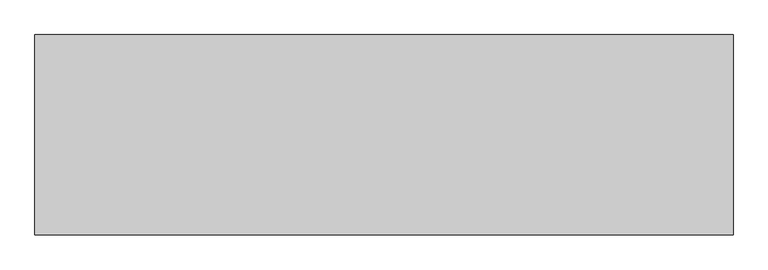
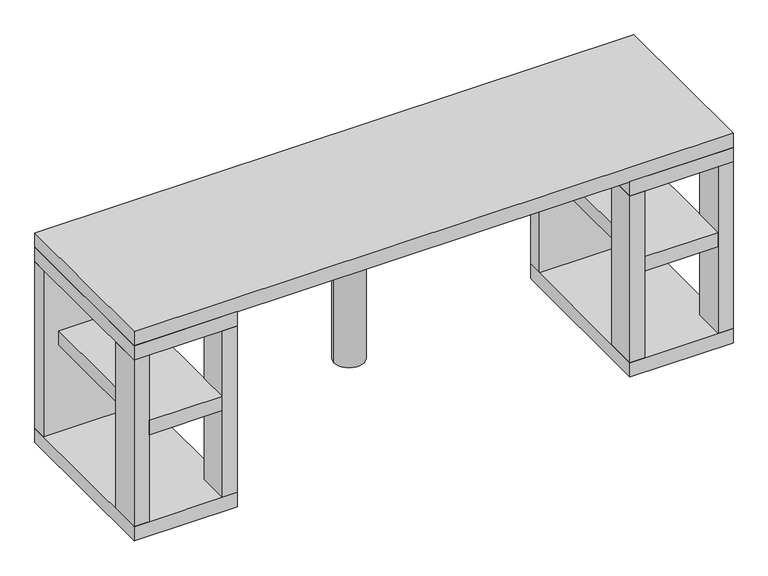
"""IFC4 building model written with IfcOpenShell, lengths in millimetres: furniture geometry."""

from ifc_helpers import new_model, si_unit, point, frame, frame_2d, origin, origin_with_axes, place, context, project, spatial, polyline, circle_curve, trimmed, segment, composite_curve, outline, extrude, source, transform, mapped, element, save


def furniture_8acf2248(model_context):
    return source(origin(), model_context, "Body", "SweptSolid", [
        extrude(outline(polyline([(349.25, 0.0), (349.25, -581.025), (0.0, -581.025), (0.0, 0.0), (349.25, 0.0)])), origin_with_axes(), (0.0, 0.0, 1.0), 50.8),
        extrude(outline(polyline([(349.25, 0.0), (349.25, -581.025), (0.0, -581.025), (0.0, 0.0), (349.25, 0.0)])), frame((0.0, 0.0, 647.7), z_axis=(0.0, 0.0, 1.0), x_axis=(1.0, 0.0, 0.0)), (0.0, 0.0, 1.0), 50.8),
        extrude(outline(polyline([(0.0, -50.8), (0.0, 0.0), (349.25, 0.0), (349.25, -50.8), (0.0, -50.8)])), frame((0.0, 0.0, 50.8), z_axis=(0.0, 0.0, 1.0), x_axis=(1.0, 0.0, 0.0)), (0.0, 0.0, 1.0), 596.9),
        extrude(outline(polyline([(298.45, -474.5110703), (349.25, -474.5110703), (349.25, -581.025), (298.45, -581.025), (298.45, -474.5110703)])), frame((0.0, 0.0, 50.8), z_axis=(0.0, 0.0, 1.0), x_axis=(1.0, 0.0, 0.0)), (0.0, 0.0, 1.0), 596.9),
        extrude(outline(polyline([(0.0, -474.5110703), (50.8, -474.5110703), (50.8, -581.025), (0.0, -581.025), (0.0, -474.5110703)])), frame((0.0, 0.0, 50.8), z_axis=(0.0, 0.0, 1.0), x_axis=(1.0, 0.0, 0.0)), (0.0, 0.0, 1.0), 596.9),
        extrude(outline(polyline([(298.45, -581.025), (50.8, -581.025), (50.8, -50.8), (298.45, -50.8), (298.45, -581.025)])), frame((0.0, 0.0, 361.95), z_axis=(0.0, 0.0, 1.0), x_axis=(1.0, 0.0, 0.0)), (0.0, 0.0, 1.0), 50.8),
        extrude(outline(polyline([(2025.65, 0.0), (2025.65, -581.025), (1676.4, -581.025), (1676.4, 0.0), (2025.65, 0.0)])), origin_with_axes(), (0.0, 0.0, 1.0), 50.8),
        extrude(outline(polyline([(2025.65, 0.0), (2025.65, -581.025), (1676.4, -581.025), (1676.4, 0.0), (2025.65, 0.0)])), frame((0.0, 0.0, 647.7), z_axis=(0.0, 0.0, 1.0), x_axis=(1.0, 0.0, 0.0)), (0.0, 0.0, 1.0), 50.8),
        extrude(outline(polyline([(1676.4, -50.8), (1676.4, 0.0), (2025.65, 0.0), (2025.65, -50.8), (1676.4, -50.8)])), frame((0.0, 0.0, 50.8), z_axis=(0.0, 0.0, 1.0), x_axis=(1.0, 0.0, 0.0)), (0.0, 0.0, 1.0), 596.9),
        extrude(outline(polyline([(1974.85, -474.5110703), (2025.65, -474.5110703), (2025.65, -581.025), (1974.85, -581.025), (1974.85, -474.5110703)])), frame((0.0, 0.0, 50.8), z_axis=(0.0, 0.0, 1.0), x_axis=(1.0, 0.0, 0.0)), (0.0, 0.0, 1.0), 596.9),
        extrude(outline(polyline([(1676.4, -474.5110703), (1727.2, -474.5110703), (1727.2, -581.025), (1676.4, -581.025), (1676.4, -474.5110703)])), frame((0.0, 0.0, 50.8), z_axis=(0.0, 0.0, 1.0), x_axis=(1.0, 0.0, 0.0)), (0.0, 0.0, 1.0), 596.9),
        extrude(outline(polyline([(1974.85, -581.025), (1727.2, -581.025), (1727.2, -50.8), (1974.85, -50.8), (1974.85, -581.025)])), frame((0.0, 0.0, 361.95), z_axis=(0.0, 0.0, 1.0), x_axis=(1.0, 0.0, 0.0)), (0.0, 0.0, 1.0), 50.8),
        extrude(outline(polyline([(0.0, -581.025), (0.0, 0.0), (2025.65, 0.0), (2025.65, -581.025), (0.0, -581.025)])), frame((0.0, 0.0, 698.5), z_axis=(0.0, 0.0, 1.0), x_axis=(1.0, 0.0, 0.0)), (0.0, 0.0, 1.0), 50.8),
        extrude(outline(composite_curve([segment(trimmed(circle_curve(frame_2d((1012.825, -85.4622102)), 50.8), [point((962.025, -85.4622102))], [point((1063.625, -85.4622102))], False, "CARTESIAN"), True, "CONTINUOUS"), segment(trimmed(circle_curve(frame_2d((1012.825, -85.4622102)), 50.8), [point((1063.625, -85.4622102))], [point((962.025, -85.4622102))], False, "CARTESIAN"), True, "CONTINUOUS")], self_intersect=False)), origin_with_axes(), (0.0, 0.0, 1.0), 698.5),
    ])


if __name__ == "__main__":
    model = new_model("IFC4")
    model_context = context("Model", 3, world=origin())
    ifc_project = project(units=[si_unit("LENGTHUNIT", "METRE", prefix="MILLI")], contexts=[model_context])
    site = spatial("IfcSite", under=ifc_project)
    building = spatial("IfcBuilding", under=site)
    placement = place(None, origin())
    furniture_shape = furniture_8acf2248(model_context)
    element("IfcFurniture", 1, at=placement, inside=building, context=model_context, shape_type="MappedRepresentation", body=[
        mapped(furniture_shape, transform((0.0, 0.0, 0.0), x_axis=(1.0, 0.0, 0.0), y_axis=(0.0, 1.0, 0.0), z_axis=(0.0, 0.0, 1.0))),
    ])
    save(model, "model.ifc")

# Revit data of these elements
# Type
#   Default Elevation = 0
